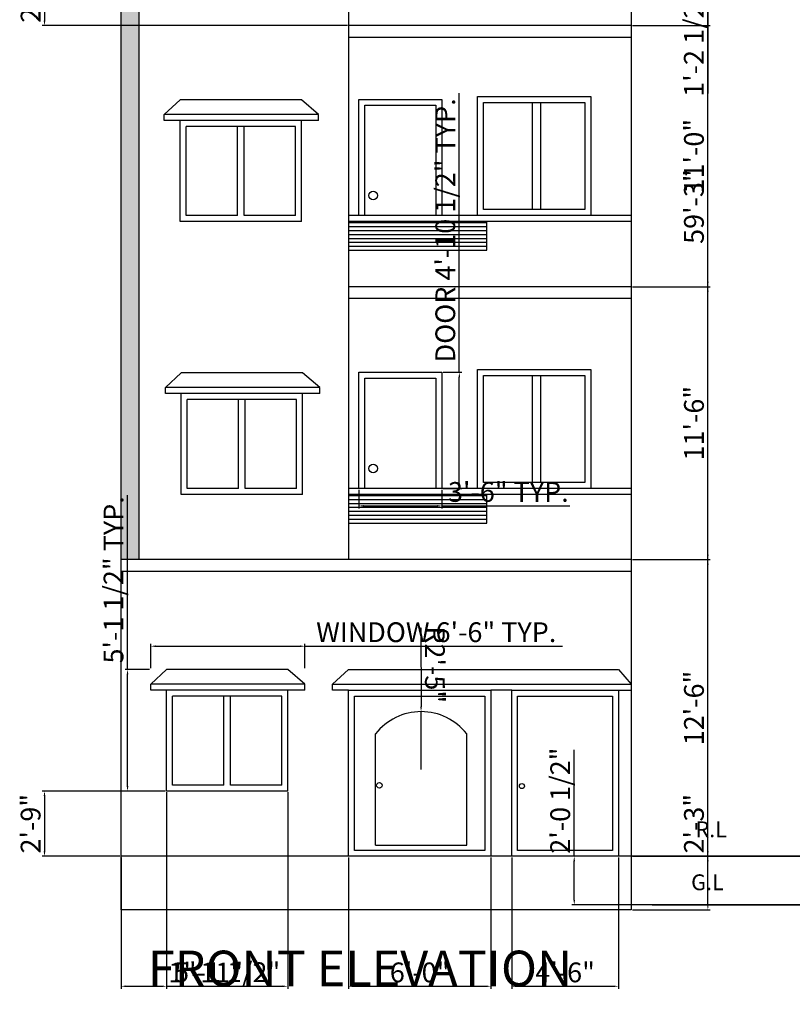
# Model space of a CAD drawing. Units: inches. Extents: x 2368 to 3882, y 1243 to 2139.
# Tile 4 of 6: x 3100 to 3491, y 1247 to 1745. Entities that reach past the tile are written whole.
import ezdxf

# ---------------------------------------------------------------- set-up
doc = ezdxf.new("R2010")
doc.units = ezdxf.units.IN
for name, color, linetype, lineweight in [('A-ANNO-DIMS', 2, 'Continuous', 18), ('A-ANNO-TEXT', 7, 'Continuous', 18), ('A-ELEV', 7, 'Continuous', 25), ('A-ELEV-PATT', 252, 'Continuous', 13), ('A-SECT', 7, 'Continuous', 35)]:
    doc.layers.add(name, color=color, linetype=linetype, lineweight=lineweight)
doc.styles.get("Standard").update_dxf_attribs({"font": 'arial.ttf'})
doc.dimstyles.new('ISO-25', dxfattribs={"dimtxt": 10, "dimasz": 2.5, "dimexe": 1.25, "dimexo": 0.625, "dimtad": 1, "dimlunit": 3, "dimtxsty": 'Standard', "dimcen": 2.5, "dimadec": 0, "dimazin": 0, "dimtfac": 1, "dimtmove": 0, "dimatfit": 3, "dimfxl": 1, "dimarcsym": 0})

# ---------------------------------------------------------------- blocks, each defined once
blk = doc.blocks.new('WIN-ELEV-CHAJJA')
for p, q in [((3166.48, 1408.84), (3174.49, 1416.36)), ((3235.8, 1416.36), (3174.49, 1416.36)), ((3244.48, 1408.84), (3235.8, 1416.36)), ((3244.48, 1408.84), (3166.48, 1408.84)), ((3166.48, 1405.84), (3166.48, 1408.84)), ((3244.48, 1405.84), (3244.48, 1408.84)), ((3244.48, 1405.84), (3166.48, 1405.84)), ((3174.49, 1354.84), (3174.49, 1405.84)), ((3235.8, 1354.84), (3235.8, 1405.84)), ((3232.8, 1402.84), (3177.49, 1402.84)), ((3177.49, 1357.84), (3177.49, 1402.84)), ((3203.49, 1357.84), (3203.49, 1402.84)), ((3206.8, 1357.84), (3206.8, 1402.84)), ((3232.8, 1357.84), (3232.8, 1402.84)), ((3235.8, 1354.84), (3174.49, 1354.84)), ((3203.49, 1357.84), (3177.49, 1357.84)), ((3232.8, 1357.84), (3206.8, 1357.84))]:
    blk.add_line(p, q)
blk = doc.blocks.new('DOOR-ELEV')
for p, q in [((3271.73, 1507.84), (3271.73, 1566.55)), ((3271.73, 1566.55), (3313.73, 1566.55)), ((3274.73, 1507.84), (3274.73, 1563.55)), ((3274.73, 1563.55), (3310.73, 1563.55)), ((3310.73, 1563.55), (3310.73, 1507.84)), ((3313.73, 1566.55), (3313.73, 1507.84))]:
    blk.add_line(p, q)
blk.add_circle((3278.95, 1517.95), 2.15)
blk = doc.blocks.new('*D20')
at = {"layer": 'A-ANNO-DIMS', "color": 0, "lineweight": -2, "transparency": 16777216}
for p, q in [((3166.48, 1416.98), (3166.48, 1429.31)), ((3244.48, 1416.98), (3244.48, 1429.31)), ((3168.98, 1428.06), (3241.98, 1428.06)), ((3244.48, 1428.06), (3374.77, 1428.06))]:
    blk.add_line(p, q, dxfattribs=at)
at = {"layer": 'A-ANNO-DIMS', "color": 0, "transparency": 16777216}
for points in [[(3168.98, 1428.48), (3168.98, 1427.64), (3166.48, 1428.06)], [(3241.98, 1428.48), (3241.98, 1427.64), (3244.48, 1428.06)]]:
    blk.add_solid(points, dxfattribs=at)
at = {"layer": 'Defpoints', "color": 0, "transparency": 16777216}
for p in [(3244.48, 1428.06), (3166.48, 1416.36), (3244.48, 1416.36)]:
    blk.add_point(p, dxfattribs=at)
at = {"layer": 'A-ANNO-DIMS', "color": 0, "transparency": 16777216, "insert": (3310.87, 1433.86), "char_height": 10, "attachment_point": 5}
blk.add_mtext('WINDOW 6\'-6" TYP.', dxfattribs=at)
blk = doc.blocks.new('*D21')
at = {"layer": 'A-ANNO-DIMS', "color": 0, "lineweight": -2, "transparency": 16777216}
for p, q in [((3154.78, 1416.36), (3154.78, 1504.37)), ((3165.85, 1416.36), (3153.53, 1416.36)), ((3154.78, 1357.34), (3154.78, 1413.86)), ((3165.85, 1354.84), (3153.53, 1354.84))]:
    blk.add_line(p, q, dxfattribs=at)
at = {"layer": 'A-ANNO-DIMS', "color": 0, "transparency": 16777216}
for points in [[(3154.36, 1413.86), (3155.19, 1413.86), (3154.78, 1416.36)], [(3154.36, 1357.34), (3155.19, 1357.34), (3154.78, 1354.84)]]:
    blk.add_solid(points, dxfattribs=at)
at = {"layer": 'Defpoints', "color": 0, "transparency": 16777216}
for p in [(3154.78, 1416.36), (3166.48, 1416.36), (3166.48, 1354.84)]:
    blk.add_point(p, dxfattribs=at)
at = {"layer": 'A-ANNO-DIMS', "color": 0, "transparency": 16777216, "insert": (3148.98, 1461.61), "char_height": 10, "attachment_point": 5, "rotation": 90}
blk.add_mtext('5\'-1 1/2" TYP.', dxfattribs=at)
blk = doc.blocks.new('*D22')
at = {"layer": 'A-ANNO-DIMS', "color": 0, "lineweight": -2, "transparency": 16777216}
for p, q in [((3322.53, 1566.55), (3322.53, 1707.62)), ((3314.35, 1566.55), (3323.78, 1566.55)), ((3322.53, 1510.34), (3322.53, 1564.05)), ((3314.35, 1507.84), (3323.78, 1507.84))]:
    blk.add_line(p, q, dxfattribs=at)
at = {"layer": 'A-ANNO-DIMS', "color": 0, "transparency": 16777216}
for points in [[(3322.12, 1564.05), (3322.95, 1564.05), (3322.53, 1566.55)], [(3322.12, 1510.34), (3322.95, 1510.34), (3322.53, 1507.84)]]:
    blk.add_solid(points, dxfattribs=at)
at = {"layer": 'Defpoints', "color": 0, "transparency": 16777216}
for p in [(3313.73, 1566.55), (3322.53, 1566.55), (3313.73, 1507.84)]:
    blk.add_point(p, dxfattribs=at)
at = {"layer": 'A-ANNO-DIMS', "color": 0, "transparency": 16777216, "insert": (3316.74, 1638.33), "char_height": 10, "attachment_point": 5, "rotation": 90}
blk.add_mtext('DOOR 4\'-10 1/2" TYP.', dxfattribs=at)
blk = doc.blocks.new('*D23')
at = {"layer": 'A-ANNO-DIMS', "color": 0, "lineweight": -2, "transparency": 16777216}
for p, q in [((3271.73, 1507.21), (3271.73, 1497.78)), ((3313.73, 1507.21), (3313.73, 1497.78)), ((3274.23, 1499.03), (3311.23, 1499.03)), ((3313.73, 1499.03), (3378.43, 1499.03))]:
    blk.add_line(p, q, dxfattribs=at)
at = {"layer": 'A-ANNO-DIMS', "color": 0, "transparency": 16777216}
for points in [[(3274.23, 1499.45), (3274.23, 1498.61), (3271.73, 1499.03)], [(3311.23, 1499.45), (3311.23, 1498.61), (3313.73, 1499.03)]]:
    blk.add_solid(points, dxfattribs=at)
at = {"layer": 'Defpoints', "color": 0, "transparency": 16777216}
for p in [(3271.73, 1507.84), (3313.73, 1507.84), (3313.73, 1499.03)]:
    blk.add_point(p, dxfattribs=at)
at = {"layer": 'A-ANNO-DIMS', "color": 0, "transparency": 16777216, "insert": (3347.33, 1504.77), "char_height": 10, "attachment_point": 5}
blk.add_mtext('3\'-6" TYP.', dxfattribs=at)
blk = doc.blocks.new('*D66')
at = {"layer": 'A-ANNO-DIMS', "color": 0, "lineweight": -2, "transparency": 16777216}
for p, q in [((3448.2, 1321.84), (3448.2, 1352.34)), ((3410.12, 1321.84), (3449.45, 1321.84)), ((3448.2, 1297.34), (3448.2, 1319.34)), ((3410.12, 1294.84), (3449.45, 1294.84))]:
    blk.add_line(p, q, dxfattribs=at)
at = {"layer": 'A-ANNO-DIMS', "color": 0, "transparency": 16777216}
for points in [[(3447.78, 1319.34), (3448.61, 1319.34), (3448.2, 1321.84)], [(3447.78, 1297.34), (3448.61, 1297.34), (3448.2, 1294.84)]]:
    blk.add_solid(points, dxfattribs=at)
at = {"layer": 'Defpoints', "color": 0, "transparency": 16777216}
for p in [(3409.5, 1321.84), (3448.2, 1321.84), (3409.5, 1294.84)]:
    blk.add_point(p, dxfattribs=at)
at = {"layer": 'A-ANNO-DIMS', "color": 0, "transparency": 16777216, "insert": (3442.46, 1338.34), "char_height": 10, "attachment_point": 5, "rotation": 90}
blk.add_mtext('2\'-3"', dxfattribs=at)
blk = doc.blocks.new('*D67')
at = {"layer": 'A-ANNO-DIMS', "color": 0, "lineweight": -2, "transparency": 16777216}
for p, q in [((3410.12, 1471.84), (3449.45, 1471.84)), ((3448.2, 1324.34), (3448.2, 1469.34)), ((3410.12, 1321.84), (3449.45, 1321.84))]:
    blk.add_line(p, q, dxfattribs=at)
at = {"layer": 'A-ANNO-DIMS', "color": 0, "transparency": 16777216}
for points in [[(3447.78, 1469.34), (3448.61, 1469.34), (3448.2, 1471.84)], [(3447.78, 1324.34), (3448.61, 1324.34), (3448.2, 1321.84)]]:
    blk.add_solid(points, dxfattribs=at)
at = {"layer": 'Defpoints', "color": 0, "transparency": 16777216}
for p in [(3409.5, 1471.84), (3448.2, 1471.84), (3409.5, 1321.84)]:
    blk.add_point(p, dxfattribs=at)
at = {"layer": 'A-ANNO-DIMS', "color": 0, "transparency": 16777216, "insert": (3442.47, 1396.84), "char_height": 10, "attachment_point": 5, "rotation": 90}
blk.add_mtext('12\'-6"', dxfattribs=at)
blk = doc.blocks.new('*D68')
at = {"layer": 'A-ANNO-DIMS', "color": 0, "lineweight": -2, "transparency": 16777216}
for p, q in [((3410.12, 1609.84), (3449.45, 1609.84)), ((3448.2, 1474.34), (3448.2, 1607.34)), ((3410.12, 1471.84), (3449.45, 1471.84))]:
    blk.add_line(p, q, dxfattribs=at)
at = {"layer": 'A-ANNO-DIMS', "color": 0, "transparency": 16777216}
for points in [[(3447.78, 1607.34), (3448.61, 1607.34), (3448.2, 1609.84)], [(3447.78, 1474.34), (3448.61, 1474.34), (3448.2, 1471.84)]]:
    blk.add_solid(points, dxfattribs=at)
at = {"layer": 'Defpoints', "color": 0, "transparency": 16777216}
for p in [(3409.5, 1609.84), (3448.2, 1609.84), (3409.5, 1471.84)]:
    blk.add_point(p, dxfattribs=at)
at = {"layer": 'A-ANNO-DIMS', "color": 0, "transparency": 16777216, "insert": (3442.47, 1540.84), "char_height": 10, "attachment_point": 5, "rotation": 90}
blk.add_mtext('11\'-6"', dxfattribs=at)
blk = doc.blocks.new('*D69')
at = {"layer": 'A-ANNO-DIMS', "color": 0, "lineweight": -2, "transparency": 16777216}
for p, q in [((3410.12, 1741.84), (3449.45, 1741.84)), ((3448.2, 1612.34), (3448.2, 1739.34)), ((3410.12, 1609.84), (3449.45, 1609.84))]:
    blk.add_line(p, q, dxfattribs=at)
at = {"layer": 'A-ANNO-DIMS', "color": 0, "transparency": 16777216}
for points in [[(3447.78, 1739.34), (3448.61, 1739.34), (3448.2, 1741.84)], [(3447.78, 1612.34), (3448.61, 1612.34), (3448.2, 1609.84)]]:
    blk.add_solid(points, dxfattribs=at)
at = {"layer": 'Defpoints', "color": 0, "transparency": 16777216}
for p in [(3409.5, 1741.84), (3448.2, 1741.84), (3409.5, 1609.84)]:
    blk.add_point(p, dxfattribs=at)
at = {"layer": 'A-ANNO-DIMS', "color": 0, "transparency": 16777216, "insert": (3442.47, 1675.84), "char_height": 10, "attachment_point": 5, "rotation": 90}
blk.add_mtext('11\'-0"', dxfattribs=at)
blk = doc.blocks.new('*D70')
at = {"layer": 'A-ANNO-DIMS', "color": 0, "lineweight": -2, "transparency": 16777216}
for p, q in [((3410.12, 1879.84), (3449.45, 1879.84)), ((3448.2, 1744.34), (3448.2, 1877.34)), ((3410.12, 1741.84), (3449.45, 1741.84))]:
    blk.add_line(p, q, dxfattribs=at)
at = {"layer": 'A-ANNO-DIMS', "color": 0, "transparency": 16777216}
for points in [[(3447.78, 1877.34), (3448.61, 1877.34), (3448.2, 1879.84)], [(3447.78, 1744.34), (3448.61, 1744.34), (3448.2, 1741.84)]]:
    blk.add_solid(points, dxfattribs=at)
at = {"layer": 'Defpoints', "color": 0, "transparency": 16777216}
for p in [(3409.5, 1879.84), (3448.2, 1879.84), (3409.5, 1741.84)]:
    blk.add_point(p, dxfattribs=at)
at = {"layer": 'A-ANNO-DIMS', "color": 0, "transparency": 16777216, "insert": (3442.47, 1810.84), "char_height": 10, "attachment_point": 5, "rotation": 90}
blk.add_mtext('11\'-6"', dxfattribs=at)
blk = doc.blocks.new('*D73')
at = {"layer": 'A-ANNO-DIMS', "color": 0, "lineweight": -2, "transparency": 16777216}
for p, q in [((3410.12, 2005.84), (3449.45, 2005.84)), ((3448.2, 1297.34), (3448.2, 2003.34)), ((3410.12, 1294.84), (3449.45, 1294.84))]:
    blk.add_line(p, q, dxfattribs=at)
at = {"layer": 'A-ANNO-DIMS', "color": 0, "transparency": 16777216}
for points in [[(3447.78, 2003.34), (3448.61, 2003.34), (3448.2, 2005.84)], [(3447.78, 1297.34), (3448.61, 1297.34), (3448.2, 1294.84)]]:
    blk.add_solid(points, dxfattribs=at)
at = {"layer": 'Defpoints', "color": 0, "transparency": 16777216}
for p in [(3409.5, 2005.84), (3448.2, 2005.84), (3409.5, 1294.84)]:
    blk.add_point(p, dxfattribs=at)
at = {"layer": 'A-ANNO-DIMS', "color": 0, "transparency": 16777216, "insert": (3442.46, 1650.34), "char_height": 10, "attachment_point": 5, "rotation": 90}
blk.add_mtext('59\'-3"', dxfattribs=at)
blk = doc.blocks.new('*D80')
at = {"layer": 'A-ANNO-DIMS', "color": 0, "lineweight": -2, "transparency": 16777216}
for p, q in [((3242.81, 1774.84), (3111.55, 1774.84)), ((3112.8, 1772.34), (3112.8, 1744.34)), ((3265.97, 1741.84), (3111.55, 1741.84))]:
    blk.add_line(p, q, dxfattribs=at)
at = {"layer": 'A-ANNO-DIMS', "color": 0, "transparency": 16777216}
for points in [[(3112.38, 1772.34), (3113.21, 1772.34), (3112.8, 1774.84)], [(3112.38, 1744.34), (3113.21, 1744.34), (3112.8, 1741.84)]]:
    blk.add_solid(points, dxfattribs=at)
at = {"layer": 'Defpoints', "color": 0, "transparency": 16777216}
for p in [(3243.43, 1774.84), (3112.8, 1741.84), (3266.59, 1741.84)]:
    blk.add_point(p, dxfattribs=at)
at = {"layer": 'A-ANNO-DIMS', "color": 0, "transparency": 16777216, "insert": (3107.07, 1758.34), "char_height": 10, "attachment_point": 5, "rotation": 90}
blk.add_mtext('2\'-9"', dxfattribs=at)
blk = doc.blocks.new('*D81')
at = {"layer": 'A-ANNO-DIMS', "color": 0, "lineweight": -2, "transparency": 16777216}
for p, q in [((3337.1, 1774.84), (3449.45, 1774.84)), ((3448.2, 1772.34), (3448.2, 1762.79)), ((3337.1, 1760.29), (3449.45, 1760.29)), ((3448.2, 1760.29), (3448.2, 1707.6))]:
    blk.add_line(p, q, dxfattribs=at)
at = {"layer": 'A-ANNO-DIMS', "color": 0, "transparency": 16777216}
for points in [[(3447.78, 1772.34), (3448.61, 1772.34), (3448.2, 1774.84)], [(3447.78, 1762.79), (3448.61, 1762.79), (3448.2, 1760.29)]]:
    blk.add_solid(points, dxfattribs=at)
at = {"layer": 'Defpoints', "color": 0, "transparency": 16777216}
for p in [(3336.47, 1774.84), (3336.47, 1760.29), (3448.2, 1760.29)]:
    blk.add_point(p, dxfattribs=at)
at = {"layer": 'A-ANNO-DIMS', "color": 0, "transparency": 16777216, "insert": (3442.4, 1732.69), "char_height": 10, "attachment_point": 5, "rotation": 90}
blk.add_mtext('1\'-2 1/2"', dxfattribs=at)
blk = doc.blocks.new('*D82')
at = {"layer": 'A-ANNO-DIMS', "color": 0, "lineweight": -2, "transparency": 16777216}
for p, q in [((3174.49, 1354.21), (3174.49, 1254.89)), ((3151.5, 1321.21), (3151.5, 1254.89)), ((3154, 1256.14), (3171.99, 1256.14)), ((3174.49, 1256.14), (3211.65, 1256.14))]:
    blk.add_line(p, q, dxfattribs=at)
at = {"layer": 'A-ANNO-DIMS', "color": 0, "transparency": 16777216}
for points in [[(3154, 1256.55), (3154, 1255.72), (3151.5, 1256.14)], [(3171.99, 1256.55), (3171.99, 1255.72), (3174.49, 1256.14)]]:
    blk.add_solid(points, dxfattribs=at)
at = {"layer": 'Defpoints', "color": 0, "transparency": 16777216}
for p in [(3174.49, 1354.84), (3151.5, 1321.84), (3174.49, 1256.14)]:
    blk.add_point(p, dxfattribs=at)
at = {"layer": 'A-ANNO-DIMS', "color": 0, "transparency": 16777216, "insert": (3194.32, 1261.78), "char_height": 10, "attachment_point": 5}
blk.add_mtext('1\'-11"', dxfattribs=at)
blk = doc.blocks.new('*D83')
at = {"layer": 'A-ANNO-DIMS', "color": 0, "lineweight": -2, "transparency": 16777216}
for p, q in [((3174.49, 1354.21), (3174.49, 1254.89)), ((3235.8, 1354.21), (3235.8, 1254.89)), ((3176.99, 1256.14), (3233.3, 1256.14))]:
    blk.add_line(p, q, dxfattribs=at)
at = {"layer": 'A-ANNO-DIMS', "color": 0, "transparency": 16777216}
for points in [[(3176.99, 1256.55), (3176.99, 1255.72), (3174.49, 1256.14)], [(3233.3, 1256.55), (3233.3, 1255.72), (3235.8, 1256.14)]]:
    blk.add_solid(points, dxfattribs=at)
at = {"layer": 'Defpoints', "color": 0, "transparency": 16777216}
for p in [(3174.49, 1354.84), (3235.8, 1354.84), (3235.8, 1256.14)]:
    blk.add_point(p, dxfattribs=at)
at = {"layer": 'A-ANNO-DIMS', "color": 0, "transparency": 16777216, "insert": (3205.15, 1261.93), "char_height": 10, "attachment_point": 5}
blk.add_mtext('5\'-1 1/2"', dxfattribs=at)
blk = doc.blocks.new('*D84')
at = {"layer": 'A-ANNO-DIMS', "color": 0, "lineweight": -2, "transparency": 16777216}
for p, q in [((3266.48, 1321.21), (3266.48, 1254.89)), ((3338.48, 1321.21), (3338.48, 1254.89)), ((3268.98, 1256.14), (3335.98, 1256.14))]:
    blk.add_line(p, q, dxfattribs=at)
at = {"layer": 'A-ANNO-DIMS', "color": 0, "transparency": 16777216}
for points in [[(3268.98, 1256.55), (3268.98, 1255.72), (3266.48, 1256.14)], [(3335.98, 1256.55), (3335.98, 1255.72), (3338.48, 1256.14)]]:
    blk.add_solid(points, dxfattribs=at)
at = {"layer": 'Defpoints', "color": 0, "transparency": 16777216}
for p in [(3266.48, 1321.84), (3338.48, 1321.84), (3338.48, 1256.14)]:
    blk.add_point(p, dxfattribs=at)
at = {"layer": 'A-ANNO-DIMS', "color": 0, "transparency": 16777216, "insert": (3302.48, 1261.87), "char_height": 10, "attachment_point": 5}
blk.add_mtext('6\'-0"', dxfattribs=at)
blk = doc.blocks.new('*D85')
at = {"layer": 'A-ANNO-DIMS', "color": 0, "lineweight": -2, "transparency": 16777216}
for p, q in [((3349.02, 1321.21), (3349.02, 1254.89)), ((3403.02, 1321.21), (3403.02, 1254.89)), ((3351.52, 1256.14), (3400.52, 1256.14))]:
    blk.add_line(p, q, dxfattribs=at)
at = {"layer": 'A-ANNO-DIMS', "color": 0, "transparency": 16777216}
for points in [[(3351.52, 1256.55), (3351.52, 1255.72), (3349.02, 1256.14)], [(3400.52, 1256.55), (3400.52, 1255.72), (3403.02, 1256.14)]]:
    blk.add_solid(points, dxfattribs=at)
at = {"layer": 'Defpoints', "color": 0, "transparency": 16777216}
for p in [(3349.02, 1321.84), (3403.02, 1321.84), (3403.02, 1256.14)]:
    blk.add_point(p, dxfattribs=at)
at = {"layer": 'A-ANNO-DIMS', "color": 0, "transparency": 16777216, "insert": (3376.02, 1261.87), "char_height": 10, "attachment_point": 5}
blk.add_mtext('4\'-6"', dxfattribs=at)
blk = doc.blocks.new('*D86')
at = {"layer": 'A-ANNO-DIMS', "color": 0, "lineweight": -2, "transparency": 16777216}
for p, q in [((3173.87, 1354.84), (3111.55, 1354.84)), ((3112.8, 1352.34), (3112.8, 1324.34)), ((3150.87, 1321.84), (3111.55, 1321.84))]:
    blk.add_line(p, q, dxfattribs=at)
at = {"layer": 'A-ANNO-DIMS', "color": 0, "transparency": 16777216}
for points in [[(3112.38, 1352.34), (3113.21, 1352.34), (3112.8, 1354.84)], [(3112.38, 1324.34), (3113.21, 1324.34), (3112.8, 1321.84)]]:
    blk.add_solid(points, dxfattribs=at)
at = {"layer": 'Defpoints', "color": 0, "transparency": 16777216}
for p in [(3174.49, 1354.84), (3112.8, 1321.84), (3151.5, 1321.84)]:
    blk.add_point(p, dxfattribs=at)
at = {"layer": 'A-ANNO-DIMS', "color": 0, "transparency": 16777216, "insert": (3107.07, 1338.34), "char_height": 10, "attachment_point": 5, "rotation": 90}
blk.add_mtext('2\'-9"', dxfattribs=at)
blk = doc.blocks.new('*D92')
at = {"layer": 'A-ANNO-DIMS', "color": 0, "lineweight": -2, "transparency": 16777216}
for p, q in [((3380.64, 1321.84), (3380.64, 1375.64)), ((3537.71, 1321.84), (3379.39, 1321.84)), ((3380.64, 1299.76), (3380.64, 1319.34)), ((3537.71, 1297.26), (3379.39, 1297.26))]:
    blk.add_line(p, q, dxfattribs=at)
at = {"layer": 'A-ANNO-DIMS', "color": 0, "transparency": 16777216}
for points in [[(3380.23, 1319.34), (3381.06, 1319.34), (3380.64, 1321.84)], [(3380.23, 1299.76), (3381.06, 1299.76), (3380.64, 1297.26)]]:
    blk.add_solid(points, dxfattribs=at)
at = {"layer": 'Defpoints', "color": 0, "transparency": 16777216}
for p in [(3380.64, 1321.84), (3538.34, 1321.84), (3538.34, 1297.26)]:
    blk.add_point(p, dxfattribs=at)
at = {"layer": 'A-ANNO-DIMS', "color": 0, "transparency": 16777216, "insert": (3374.85, 1349.99), "char_height": 10, "attachment_point": 5, "rotation": 90}
blk.add_mtext('2\'-0 1/2"', dxfattribs=at)
blk = doc.blocks.new('*D97')
at = {"layer": 'A-ANNO-DIMS', "color": 0, "lineweight": -2, "transparency": 16777216}
for p, q in [((3303.14, 1437.39), (3303.2, 1397.49)), ((3303.24, 1365.75), (3303.2, 1394.99))]:
    blk.add_line(p, q, dxfattribs=at)
at = {"layer": 'A-ANNO-DIMS', "color": 0, "transparency": 16777216}
blk.add_solid([(3303.61, 1397.49), (3302.78, 1397.49), (3303.2, 1394.99)], dxfattribs=at)
at = {"layer": 'Defpoints', "color": 0, "transparency": 16777216}
for p in [(3303.2, 1394.99), (3303.24, 1365.75)]:
    blk.add_point(p, dxfattribs=at)
at = {"layer": 'A-ANNO-DIMS', "color": 0, "transparency": 16777216, "insert": (3308.9, 1418.7), "char_height": 10, "attachment_point": 5, "rotation": 270.0773}
blk.add_mtext('R2\'-5"', dxfattribs=at)

msp = doc.modelspace()

# ---------------------------------------------------------------- hatches: boundary and pattern name
at = {"layer": 'A-ELEV-PATT'}
h = msp.add_hatch(dxfattribs=at)
h.set_pattern_fill('AR-CONC', color=256, scale=0.066)
h.paths.add_polyline_path([(3409.496, 1921.838), (3151.496, 1921.838), (3151.496, 1471.838), (3160.496, 1471.838), (3160.496, 1909.838), (3400.496, 1909.838), (3400.496, 1879.838), (3409.496, 1879.838)])

# ---------------------------------------------------------------- linework, layer by layer
at = {"layer": 'A-ELEV'}
for p, q in [((3151.496, 1294.838), (3151.496, 1921.838)), ((3409.496, 1921.838), (3409.496, 1294.838)), ((3160.496, 1909.838), (3160.496, 1471.838)), ((3266.593, 1471.838), (3266.593, 1873.838)), ((3409.496, 1741.838), (3266.593, 1741.838)), ((3409.496, 1735.838), (3266.593, 1735.838)), ((3359.418, 1703.025), (3359.418, 1648.838)), ((3363.593, 1703.025), (3363.593, 1648.838)), ((3409.496, 1645.838), (3266.593, 1645.838)), ((3409.496, 1642.838), (3266.593, 1642.838)), ((3336.475, 1628.289), (3336.475, 1642.838)), ((3266.593, 1642.289), (3336.475, 1642.289)), ((3266.593, 1640.289), (3336.475, 1640.289)), ((3266.593, 1638.289), (3336.475, 1638.289)), ((3266.593, 1636.289), (3336.475, 1636.289)), ((3266.593, 1634.289), (3336.475, 1634.289)), ((3266.593, 1632.289), (3336.475, 1632.289)), ((3266.593, 1630.289), (3336.475, 1630.289)), ((3266.593, 1628.289), (3336.475, 1628.289)), ((3409.496, 1609.838), (3266.593, 1609.838)), ((3409.496, 1603.838), (3266.593, 1603.838)), ((3359.418, 1565.025), (3359.418, 1510.838)), ((3363.593, 1565.025), (3363.593, 1510.838)), ((3409.496, 1507.838), (3266.593, 1507.838)), ((3409.496, 1504.838), (3266.593, 1504.838)), ((3266.593, 1504.289), (3336.475, 1504.289)), ((3336.475, 1490.289), (3336.475, 1504.838)), ((3266.593, 1502.289), (3336.475, 1502.289)), ((3266.593, 1500.289), (3336.475, 1500.289)), ((3266.593, 1498.289), (3336.475, 1498.289)), ((3266.593, 1496.289), (3336.475, 1496.289)), ((3266.593, 1494.289), (3336.475, 1494.289)), ((3266.593, 1492.289), (3336.475, 1492.289)), ((3266.593, 1490.289), (3336.475, 1490.289)), ((3409.496, 1471.838), (3151.496, 1471.838)), ((3409.496, 1465.838), (3151.496, 1465.838)), ((3266.479, 1416.359), (3258.479, 1408.838)), ((3266.479, 1416.359), (3403.023, 1416.359)), ((3403.023, 1416.359), (3409.496, 1408.838)), ((3258.479, 1405.838), (3258.479, 1408.838)), ((3258.479, 1408.838), (3409.496, 1408.838)), ((3266.479, 1405.838), (3258.479, 1405.838)), ((3349.023, 1405.838), (3338.479, 1405.838)), ((3403.023, 1405.838), (3409.496, 1405.838)), ((3280.212, 1327.411), (3280.212, 1383.764)), ((3326.267, 1327.411), (3326.267, 1383.764)), ((3280.212, 1327.411), (3326.267, 1327.411)), ((3409.496, 1321.838), (3151.496, 1321.838)), ((3409.496, 1294.838), (3151.496, 1294.838))]:
    msp.add_line(p, q, dxfattribs=at)
for points in [[(3331.795, 1706.025), (3389.041, 1706.025), (3389.041, 1645.838), (3331.795, 1645.838)], [(3334.795, 1703.025), (3386.041, 1703.025), (3386.041, 1648.838), (3334.795, 1648.838)], [(3331.795, 1568.025), (3389.041, 1568.025), (3389.041, 1507.838), (3331.795, 1507.838)], [(3334.795, 1565.025), (3386.041, 1565.025), (3386.041, 1510.838), (3334.795, 1510.838)], [(3338.479, 1321.838), (3266.479, 1321.838), (3266.479, 1405.838), (3338.479, 1405.838)], [(3403.023, 1321.838), (3349.023, 1321.838), (3349.023, 1405.838), (3403.023, 1405.838)], [(3335.479, 1324.838), (3269.479, 1324.838), (3269.479, 1402.838), (3335.479, 1402.838)], [(3400.023, 1324.838), (3352.023, 1324.838), (3352.023, 1402.838), (3400.023, 1402.838)]]:
    msp.add_lwpolyline(points, close=True, dxfattribs=at)
for centre, radius in [((3282.111, 1357.751), 1.404), ((3354.218, 1357.372), 1.286)]:
    msp.add_circle(centre, radius, dxfattribs=at)
msp.add_arc((3303.239, 1365.749), 29.238, 38.03725, 141.96275, dxfattribs=at)
at = {"layer": 'A-SECT'}
for p, q in [((3538.338, 1321.838), (3419.342, 1321.838)), ((3538.338, 1297.261), (3420.08, 1297.261))]:
    msp.add_line(p, q, dxfattribs=at)

# ---------------------------------------------------------------- block references
at = {"layer": 'A-ELEV'}
for name, p in [('WIN-ELEV-CHAJJA', (6.89, 288)), ('DOOR-ELEV', (0, 138)), ('WIN-ELEV-CHAJJA', (7.448, 150)), ('DOOR-ELEV', (0, 0)), ('WIN-ELEV-CHAJJA', (0, 0))]:
    msp.add_blockref(name, p, dxfattribs=at)

# ---------------------------------------------------------------- texts
at = {"layer": 'A-ANNO-TEXT'}
for s, height, p in [('R.L', 8, (3441.962, 1331.49)), ('G.L', 8, (3439.75, 1304.714)), ('FRONT ELEVATION ', 18, (3165.059, 1256.145))]:
    msp.add_text(s, height=height, dxfattribs=at).set_placement(p)

# ---------------------------------------------------------------- dimensions: what is measured, and where the dimension line sits
at = {"layer": 'A-ANNO-DIMS'}
for base, p1, p2, picture, middle in [((3448.196, 2005.838), (3409.496, 1294.838), (3409.496, 2005.838), '*D73', (3442.462, 1650.338)), ((3448.196, 1879.838), (3409.496, 1741.838), (3409.496, 1879.838), '*D70', (3442.466, 1810.838)), ((3112.796, 1741.838), (3243.431, 1774.838), (3266.593, 1741.838), '*D80', (3107.066, 1758.338)), ((3448.196, 1760.289), (3336.475, 1774.838), (3336.475, 1760.289), '*D81', (3442.401, 1732.692)), ((3448.196, 1741.838), (3409.496, 1609.838), (3409.496, 1741.838), '*D69', (3442.466, 1675.838)), ((3448.196, 1609.838), (3409.496, 1471.838), (3409.496, 1609.838), '*D68', (3442.466, 1540.838)), ((3448.196, 1471.838), (3409.496, 1321.838), (3409.496, 1471.838), '*D67', (3442.466, 1396.838)), ((3380.642, 1321.838), (3538.338, 1297.261), (3538.338, 1321.838), '*D92', (3374.847, 1349.99)), ((3112.796, 1321.838), (3174.493, 1354.838), (3151.496, 1321.838), '*D86', (3107.066, 1338.338)), ((3448.196, 1321.838), (3409.496, 1294.838), (3409.496, 1321.838), '*D66', (3442.462, 1338.339))]:
    dim = msp.add_linear_dim(base=base, p1=p1, p2=p2, angle=90, dimstyle='ISO-25', override={"dimdec": 1, "dimlfac": 1, "dimrnd": 0, "dimzin": 1, "dimdsep": 46, "dimlunit": 4, "dimfrac": 2}, dxfattribs=at)
    dim.commit()
    dim.dimension.update_dxf_attribs({"geometry": picture, "text_midpoint": middle})
for base, p1, p2, text, picture, middle in [((3322.534, 1566.546), (3313.728, 1507.838), (3313.728, 1566.546), 'DOOR <> TYP.', '*D22', (3316.735, 1638.33)), ((3154.776, 1416.359), (3166.476, 1354.838), (3166.476, 1416.359), '<> TYP.', '*D21', (3148.98, 1461.612))]:
    dim = msp.add_linear_dim(base=base, p1=p1, p2=p2, angle=90, text=text, dimstyle='ISO-25', override={"dimdec": 1, "dimrnd": 0, "dimzin": 1, "dimlunit": 4, "dimfrac": 2}, dxfattribs=at)
    dim.commit()
    dim.dimension.update_dxf_attribs({"geometry": picture, "text_midpoint": middle})
for base, p1, p2, text, picture, middle in [((3313.728, 1499.031), (3271.728, 1507.838), (3313.728, 1507.838), '<> TYP.', '*D23', (3347.327, 1504.766)), ((3244.476, 1428.059), (3166.476, 1416.359), (3244.476, 1416.359), 'WINDOW <> TYP.', '*D20', (3310.872, 1433.858))]:
    dim = msp.add_linear_dim(base=base, p1=p1, p2=p2, text=text, dimstyle='ISO-25', override={"dimdec": 1, "dimrnd": 0, "dimzin": 1, "dimlunit": 4, "dimfrac": 2}, dxfattribs=at)
    dim.commit()
    dim.dimension.update_dxf_attribs({"geometry": picture, "text_midpoint": middle})
dim = msp.add_radius_dim(center=(3303.239, 1365.749), mpoint=(3303.2, 1394.986), dimstyle='ISO-25', override={"dimdec": 1, "dimlfac": 1, "dimrnd": 0, "dimzin": 1, "dimdsep": 46, "dimlunit": 4, "dimfrac": 2}, dxfattribs=at)
dim.commit()
dim.dimension.update_dxf_attribs({"geometry": '*D97', "text_midpoint": (3308.899, 1418.695)})
for base, p1, p2, picture, middle in [((3174.493, 1256.138), (3151.496, 1321.838), (3174.493, 1354.838), '*D82', (3194.324, 1261.783)), ((3235.804, 1256.138), (3174.493, 1354.838), (3235.804, 1354.838), '*D83', (3205.149, 1261.933)), ((3338.479, 1256.138), (3266.479, 1321.838), (3338.479, 1321.838), '*D84', (3302.479, 1261.868)), ((3403.023, 1256.138), (3349.023, 1321.838), (3403.023, 1321.838), '*D85', (3376.023, 1261.868))]:
    dim = msp.add_linear_dim(base=base, p1=p1, p2=p2, dimstyle='ISO-25', override={"dimdec": 1, "dimlfac": 1, "dimrnd": 0, "dimzin": 1, "dimdsep": 46, "dimlunit": 4, "dimfrac": 2}, dxfattribs=at)
    dim.commit()
    dim.dimension.update_dxf_attribs({"geometry": picture, "text_midpoint": middle})

doc.saveas('drawing.dxf')
